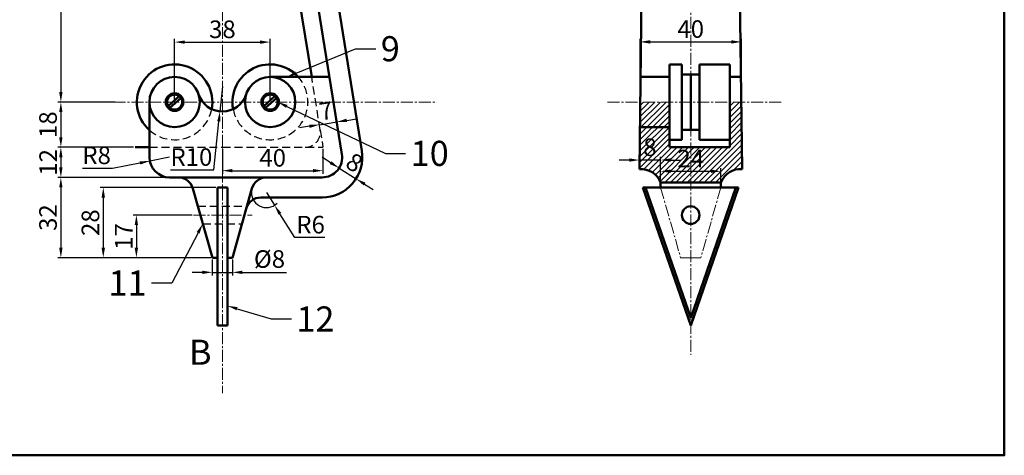
# Model space of a CAD drawing. Units: millimetres. Extents: x 376 to 1043, y -28 to 427.
# Tile 4 of 5: x 651 to 1043, y -28 to 145. Entities that reach past the tile are written whole.
import ezdxf
from ezdxf import colors
from ezdxf.entities.mleader import LeaderData, LeaderLine
from ezdxf.math import Vec2, Vec3

# ---------------------------------------------------------------- set-up
doc = ezdxf.new("R2010")
doc.units = ezdxf.units.MM
doc.header["$LTSCALE"] = 0.5
doc.linetypes.add('CENTER2', pattern=[28.575, 19.05, -3.175, 3.175, -3.175])
doc.linetypes.add('DASHED', pattern=[19.05, 12.7, -6.35])
for name, color, linetype, lineweight in [('M-CNTR', 1, 'CENTER2', 18), ('M-DIMS', 2, 'Continuous', 25), ('M-HATC', 8, 'Continuous', 18), ('M-HIDN', 4, 'DASHED', 25), ('M-OUTL', 7, 'Continuous', 50), ('M-TEXT', 7, 'Continuous', 25)]:
    doc.layers.add(name, color=color, linetype=linetype, lineweight=lineweight)
doc.styles.get("Standard").update_dxf_attribs({"font": 'arial.ttf'})
doc.dimstyles.new('ISO-25', dxfattribs={"dimtxt": 7, "dimasz": 4, "dimexe": 1.25, "dimexo": 0.625, "dimtad": 1, "dimtoh": 1, "dimtxsty": 'Standard', "dimcen": 2.5, "dimadec": 0, "dimazin": 0, "dimtfac": 1, "dimtmove": 0, "dimatfit": 3, "dimfxl": 1, "dimarcsym": 0})

# ---------------------------------------------------------------- blocks, each defined once
blk = doc.blocks.new('*D63')
at = {"layer": 'Defpoints', "color": 0, "ltscale": 0.5, "transparency": 16777216}
for p in [(689.88, 200.26), (667.7, 112.26), (689.88, 112.26)]:
    blk.add_point(p, dxfattribs=at)
at = {"layer": 'M-DIMS', "color": 0, "lineweight": -2, "ltscale": 0.5, "transparency": 16777216}
for p, q in [((689.26, 200.26), (666.45, 200.26)), ((667.7, 196.26), (667.7, 116.26)), ((689.26, 112.26), (666.45, 112.26))]:
    blk.add_line(p, q, dxfattribs=at)
at = {"layer": 'M-DIMS', "color": 0, "ltscale": 0.5, "transparency": 16777216}
for points in [[(667.03, 196.26), (668.37, 196.26), (667.7, 200.26)], [(667.03, 116.26), (668.37, 116.26), (667.7, 112.26)]]:
    blk.add_solid(points, dxfattribs=at)
at = {"layer": 'M-DIMS', "color": 0, "ltscale": 0.5, "transparency": 16777216, "insert": (663.5, 156.26), "char_height": 7, "attachment_point": 5, "rotation": 90}
blk.add_mtext('88', dxfattribs=at)
blk = doc.blocks.new('*D64')
at = {"layer": 'Defpoints', "color": 0, "ltscale": 0.5, "transparency": 16777216}
for p in [(689.88, 112.26), (667.7, 94.26), (697.2, 94.26)]:
    blk.add_point(p, dxfattribs=at)
at = {"layer": 'M-DIMS', "color": 0, "lineweight": -2, "ltscale": 0.5, "transparency": 16777216}
for p, q in [((689.26, 112.26), (666.45, 112.26)), ((667.7, 108.26), (667.7, 98.26)), ((696.58, 94.26), (666.45, 94.26))]:
    blk.add_line(p, q, dxfattribs=at)
at = {"layer": 'M-DIMS', "color": 0, "ltscale": 0.5, "transparency": 16777216}
for points in [[(667.03, 108.26), (668.37, 108.26), (667.7, 112.26)], [(667.03, 98.26), (668.37, 98.26), (667.7, 94.26)]]:
    blk.add_solid(points, dxfattribs=at)
at = {"layer": 'M-DIMS', "color": 0, "ltscale": 0.5, "transparency": 16777216, "insert": (663.5, 103.26), "char_height": 7, "attachment_point": 5, "rotation": 90}
blk.add_mtext('18', dxfattribs=at)
blk = doc.blocks.new('*D65')
at = {"layer": 'Defpoints', "color": 0, "ltscale": 0.5, "transparency": 16777216}
for p in [(691.58, 94.26), (667.7, 82.26), (724.71, 82.26)]:
    blk.add_point(p, dxfattribs=at)
at = {"layer": 'M-DIMS', "color": 0, "lineweight": -2, "ltscale": 0.5, "transparency": 16777216}
for p, q in [((690.96, 94.26), (666.45, 94.26)), ((667.7, 90.26), (667.7, 86.26)), ((724.08, 82.26), (666.45, 82.26))]:
    blk.add_line(p, q, dxfattribs=at)
at = {"layer": 'M-DIMS', "color": 0, "ltscale": 0.5, "transparency": 16777216}
for points in [[(667.03, 90.26), (668.37, 90.26), (667.7, 94.26)], [(667.03, 86.26), (668.37, 86.26), (667.7, 82.26)]]:
    blk.add_solid(points, dxfattribs=at)
at = {"layer": 'M-DIMS', "color": 0, "ltscale": 0.5, "transparency": 16777216, "insert": (663.56, 88.26), "char_height": 7, "attachment_point": 5, "rotation": 90}
blk.add_mtext('12', dxfattribs=at)
blk = doc.blocks.new('*D66')
at = {"layer": 'Defpoints', "color": 0, "ltscale": 0.5, "transparency": 16777216}
for p in [(684.99, 82.26), (667.7, 50.26), (727.94, 50.26)]:
    blk.add_point(p, dxfattribs=at)
at = {"layer": 'M-DIMS', "color": 0, "lineweight": -2, "ltscale": 0.5, "transparency": 16777216}
for p, q in [((684.37, 82.26), (666.45, 82.26)), ((667.7, 78.26), (667.7, 54.26)), ((727.32, 50.26), (666.45, 50.26))]:
    blk.add_line(p, q, dxfattribs=at)
at = {"layer": 'M-DIMS', "color": 0, "ltscale": 0.5, "transparency": 16777216}
for points in [[(667.03, 78.26), (668.37, 78.26), (667.7, 82.26)], [(667.03, 54.26), (668.37, 54.26), (667.7, 50.26)]]:
    blk.add_solid(points, dxfattribs=at)
at = {"layer": 'M-DIMS', "color": 0, "ltscale": 0.5, "transparency": 16777216, "insert": (663.5, 66.26), "char_height": 7, "attachment_point": 5, "rotation": 90}
blk.add_mtext('32', dxfattribs=at)
blk = doc.blocks.new('*D67')
at = {"layer": 'Defpoints', "color": 0, "ltscale": 0.5, "transparency": 16777216}
for p in [(729.94, 78.26), (684.57, 50.26), (717.58, 50.26)]:
    blk.add_point(p, dxfattribs=at)
at = {"layer": 'M-DIMS', "color": 0, "lineweight": -2, "ltscale": 0.5, "transparency": 16777216}
for p, q in [((729.32, 78.26), (683.32, 78.26)), ((684.57, 74.26), (684.57, 54.26)), ((716.96, 50.26), (683.32, 50.26))]:
    blk.add_line(p, q, dxfattribs=at)
at = {"layer": 'M-DIMS', "color": 0, "ltscale": 0.5, "transparency": 16777216}
for points in [[(683.9, 74.26), (685.24, 74.26), (684.57, 78.26)], [(683.9, 54.26), (685.24, 54.26), (684.57, 50.26)]]:
    blk.add_solid(points, dxfattribs=at)
at = {"layer": 'M-DIMS', "color": 0, "ltscale": 0.5, "transparency": 16777216, "insert": (680.37, 64.26), "char_height": 7, "attachment_point": 5, "rotation": 90}
blk.add_mtext('28', dxfattribs=at)
blk = doc.blocks.new('*D68')
at = {"layer": 'Defpoints', "color": 0, "ltscale": 0.5, "transparency": 16777216}
for p in [(720.49, 67.26), (697.74, 50.26), (717.58, 50.26)]:
    blk.add_point(p, dxfattribs=at)
at = {"layer": 'M-DIMS', "color": 0, "lineweight": -2, "ltscale": 0.5, "transparency": 16777216}
for p, q in [((719.87, 67.26), (696.49, 67.26)), ((697.74, 63.26), (697.74, 54.26)), ((716.96, 50.26), (696.49, 50.26))]:
    blk.add_line(p, q, dxfattribs=at)
at = {"layer": 'M-DIMS', "color": 0, "ltscale": 0.5, "transparency": 16777216}
for points in [[(697.07, 63.26), (698.4, 63.26), (697.74, 67.26)], [(697.07, 54.26), (698.4, 54.26), (697.74, 50.26)]]:
    blk.add_solid(points, dxfattribs=at)
at = {"layer": 'M-DIMS', "color": 0, "ltscale": 0.5, "transparency": 16777216, "insert": (693.6, 58.76), "char_height": 7, "attachment_point": 5, "rotation": 90}
blk.add_mtext('17', dxfattribs=at)
blk = doc.blocks.new('*D69')
at = {"layer": 'Defpoints', "color": 0, "ltscale": 0.5, "transparency": 16777216}
for p in [(727.94, 50.26), (735.94, 50.26), (735.94, 44.47)]:
    blk.add_point(p, dxfattribs=at)
at = {"layer": 'M-DIMS', "color": 0, "lineweight": -2, "ltscale": 0.5, "transparency": 16777216}
for p, q in [((727.94, 49.64), (727.94, 43.22)), ((735.94, 49.64), (735.94, 43.22)), ((723.94, 44.47), (719.94, 44.47)), ((727.94, 44.47), (735.94, 44.47)), ((739.94, 44.47), (757.41, 44.47))]:
    blk.add_line(p, q, dxfattribs=at)
at = {"layer": 'M-DIMS', "color": 0, "ltscale": 0.5, "transparency": 16777216}
for points in [[(723.94, 45.14), (723.94, 43.8), (727.94, 44.47)], [(739.94, 45.14), (739.94, 43.8), (735.94, 44.47)]]:
    blk.add_solid(points, dxfattribs=at)
at = {"layer": 'M-DIMS', "color": 0, "ltscale": 0.5, "transparency": 16777216, "insert": (750.68, 48.87), "char_height": 7, "attachment_point": 5}
blk.add_mtext('%%C8', dxfattribs=at)
blk = doc.blocks.new('*D70')
at = {"layer": 'Defpoints', "color": 0, "ltscale": 0.5, "transparency": 16777216}
for p in [(710.94, 90.26), (703.08, 88.78)]:
    blk.add_point(p, dxfattribs=at)
at = {"layer": 'M-DIMS', "color": 0, "lineweight": -2, "ltscale": 0.5, "transparency": 16777216}
for p, q in [((710.94, 90.26), (703.08, 88.78)), ((688.2, 85.96), (699.15, 88.03)), ((676.27, 85.96), (688.2, 85.96))]:
    blk.add_line(p, q, dxfattribs=at)
at = {"layer": 'M-DIMS', "color": 0, "ltscale": 0.5, "transparency": 16777216}
blk.add_solid([(699.03, 88.69), (699.28, 87.38), (703.08, 88.78)], dxfattribs=at)
at = {"layer": 'M-DIMS', "color": 0, "ltscale": 0.5, "transparency": 16777216, "insert": (681.92, 90.16), "char_height": 7, "attachment_point": 5}
blk.add_mtext('R8', dxfattribs=at)
blk = doc.blocks.new('*D71')
at = {"layer": 'Defpoints', "color": 0, "ltscale": 0.5, "transparency": 16777216}
for p in [(731.94, 94.26), (771.94, 94.26), (771.94, 84.95)]:
    blk.add_point(p, dxfattribs=at)
at = {"layer": 'M-DIMS', "color": 0, "lineweight": -2, "ltscale": 0.5, "transparency": 16777216}
for p, q in [((731.94, 93.64), (731.94, 83.7)), ((771.94, 93.64), (771.94, 83.7)), ((735.94, 84.95), (767.94, 84.95))]:
    blk.add_line(p, q, dxfattribs=at)
at = {"layer": 'M-DIMS', "color": 0, "ltscale": 0.5, "transparency": 16777216}
for points in [[(735.94, 85.61), (735.94, 84.28), (731.94, 84.95)], [(767.94, 85.61), (767.94, 84.28), (771.94, 84.95)]]:
    blk.add_solid(points, dxfattribs=at)
at = {"layer": 'M-DIMS', "color": 0, "ltscale": 0.5, "transparency": 16777216, "insert": (751.94, 89.15), "char_height": 7, "attachment_point": 5}
blk.add_mtext('40', dxfattribs=at)
blk = doc.blocks.new('*D72')
at = {"layer": 'Defpoints', "color": 0, "ltscale": 0.5, "transparency": 16777216}
for p in [(750.94, 136.13), (712.94, 112.26), (750.94, 112.26)]:
    blk.add_point(p, dxfattribs=at)
at = {"layer": 'M-DIMS', "color": 0, "lineweight": -2, "ltscale": 0.5, "transparency": 16777216}
for p, q in [((712.94, 112.89), (712.94, 137.38)), ((750.94, 112.89), (750.94, 137.38)), ((716.94, 136.13), (746.94, 136.13))]:
    blk.add_line(p, q, dxfattribs=at)
at = {"layer": 'M-DIMS', "color": 0, "ltscale": 0.5, "transparency": 16777216}
for points in [[(716.94, 136.79), (716.94, 135.46), (712.94, 136.13)], [(746.94, 136.79), (746.94, 135.46), (750.94, 136.13)]]:
    blk.add_solid(points, dxfattribs=at)
at = {"layer": 'M-DIMS', "color": 0, "ltscale": 0.5, "transparency": 16777216, "insert": (731.94, 140.33), "char_height": 7, "attachment_point": 5}
blk.add_mtext('38', dxfattribs=at)
blk = doc.blocks.new('*D73')
at = {"layer": 'Defpoints', "color": 0, "ltscale": 0.5, "transparency": 16777216}
for p in [(731.94, 118.51), (730.94, 108.56)]:
    blk.add_point(p, dxfattribs=at)
at = {"layer": 'M-DIMS', "color": 0, "lineweight": -2, "ltscale": 0.5, "transparency": 16777216}
for p, q in [((731.94, 118.51), (730.94, 108.56)), ((728.6, 85.26), (730.54, 104.58)), ((711.27, 85.26), (728.6, 85.26))]:
    blk.add_line(p, q, dxfattribs=at)
at = {"layer": 'M-DIMS', "color": 0, "ltscale": 0.5, "transparency": 16777216}
blk.add_solid([(729.88, 104.65), (731.2, 104.51), (730.94, 108.56)], dxfattribs=at)
at = {"layer": 'M-DIMS', "color": 0, "ltscale": 0.5, "transparency": 16777216, "insert": (719.62, 89.45), "char_height": 7, "attachment_point": 5}
blk.add_mtext('R10', dxfattribs=at)
blk = doc.blocks.new('*D74')
at = {"layer": 'Defpoints', "color": 0, "ltscale": 0.5, "transparency": 16777216}
for p in [(778.34, 86), (785.11, 81.73), (785.11, 81.73)]:
    blk.add_point(p, dxfattribs=at)
at = {"layer": 'M-DIMS', "color": 0, "lineweight": -2, "ltscale": 0.5, "transparency": 16777216}
for p, q in [((774.96, 88.13), (771.57, 90.26)), ((778.01, 85.47), (777.67, 84.94)), ((778.34, 86), (785.11, 81.73)), ((785.44, 82.26), (785.77, 82.79)), ((788.49, 79.6), (791.87, 77.47))]:
    blk.add_line(p, q, dxfattribs=at)
at = {"layer": 'M-DIMS', "color": 0, "ltscale": 0.5, "transparency": 16777216}
for points in [[(775.31, 88.7), (774.6, 87.57), (778.34, 86)], [(788.85, 80.16), (788.14, 79.04), (785.11, 81.73)]]:
    blk.add_solid(points, dxfattribs=at)
at = {"layer": 'M-DIMS', "color": 0, "ltscale": 0.5, "transparency": 16777216, "insert": (783.96, 87.42), "char_height": 7, "attachment_point": 5, "rotation": 327.7752}
blk.add_mtext('8', dxfattribs=at)
blk = doc.blocks.new('*D75')
at = {"layer": 'Defpoints', "color": 0, "ltscale": 0.5, "transparency": 16777216}
for p in [(770.5, 103.23), (777.42, 104.34), (777.42, 104.34)]:
    blk.add_point(p, dxfattribs=at)
at = {"layer": 'M-DIMS', "color": 0, "lineweight": -2, "ltscale": 0.5, "transparency": 16777216}
for p, q in [((766.56, 102.6), (762.61, 101.96)), ((770.41, 103.85), (770.31, 104.46)), ((770.5, 103.23), (777.42, 104.34)), ((777.32, 104.96), (777.22, 105.57)), ((781.37, 104.97), (785.32, 105.61))]:
    blk.add_line(p, q, dxfattribs=at)
at = {"layer": 'M-DIMS', "color": 0, "ltscale": 0.5, "transparency": 16777216}
for points in [[(766.45, 103.25), (766.66, 101.94), (770.5, 103.23)], [(781.26, 105.63), (781.47, 104.31), (777.42, 104.34)]]:
    blk.add_solid(points, dxfattribs=at)
at = {"layer": 'M-DIMS', "color": 0, "ltscale": 0.5, "transparency": 16777216, "insert": (773.31, 107.86), "char_height": 7, "attachment_point": 5, "rotation": 9.1114}
blk.add_mtext('7', dxfattribs=at)
blk = doc.blocks.new('*D81')
at = {"layer": 'Defpoints', "color": 0, "ltscale": 0.5, "transparency": 16777216}
for p in [(749.49, 76.26), (752.68, 71.19)]:
    blk.add_point(p, dxfattribs=at)
at = {"layer": 'M-DIMS', "color": 0, "lineweight": -2, "ltscale": 0.5, "transparency": 16777216}
for p, q in [((749.49, 76.26), (752.68, 71.19)), ((760.75, 58.36), (754.81, 67.8)), ((772.66, 58.36), (760.75, 58.36))]:
    blk.add_line(p, q, dxfattribs=at)
blk.add_arc((749.49, 76.26), 6, 170.2597, 314.1138, dxfattribs=at)
at = {"layer": 'M-DIMS', "color": 0, "ltscale": 0.5, "transparency": 16777216}
blk.add_solid([(755.38, 68.16), (754.25, 67.45), (752.68, 71.19)], dxfattribs=at)
at = {"layer": 'M-DIMS', "color": 0, "ltscale": 0.5, "transparency": 16777216, "insert": (767.02, 62.56), "char_height": 7, "attachment_point": 5}
blk.add_mtext('R6', dxfattribs=at)
blk = doc.blocks.new('*D85')
at = {"layer": 'Defpoints', "color": 0, "ltscale": 0.5, "transparency": 16777216}
for p in [(930.2, 84.71), (906.2, 78.26), (930.2, 78.26)]:
    blk.add_point(p, dxfattribs=at)
at = {"layer": 'M-DIMS', "color": 0, "lineweight": -2, "ltscale": 0.5, "transparency": 16777216}
for p, q in [((906.2, 78.89), (906.2, 85.96)), ((910.2, 84.71), (926.2, 84.71)), ((930.2, 78.89), (930.2, 85.96))]:
    blk.add_line(p, q, dxfattribs=at)
at = {"layer": 'M-DIMS', "color": 0, "ltscale": 0.5, "transparency": 16777216}
for points in [[(910.2, 85.38), (910.2, 84.04), (906.2, 84.71)], [(926.2, 85.38), (926.2, 84.04), (930.2, 84.71)]]:
    blk.add_solid(points, dxfattribs=at)
at = {"layer": 'M-DIMS', "color": 0, "ltscale": 0.5, "transparency": 16777216, "insert": (918.2, 88.85), "char_height": 7, "attachment_point": 5}
blk.add_mtext('24', dxfattribs=at)
blk = doc.blocks.new('*D86')
at = {"layer": 'Defpoints', "color": 0, "ltscale": 0.5, "transparency": 16777216}
for p in [(897.77, 89.18), (897.77, 85.57), (906.2, 80.26)]:
    blk.add_point(p, dxfattribs=at)
at = {"layer": 'M-DIMS', "color": 0, "lineweight": -2, "ltscale": 0.5, "transparency": 16777216}
for p, q in [((897.77, 86.19), (897.77, 90.43)), ((906.2, 80.89), (906.2, 90.43)), ((893.77, 89.18), (889.77, 89.18)), ((906.2, 89.18), (897.77, 89.18)), ((910.2, 89.18), (914.2, 89.18))]:
    blk.add_line(p, q, dxfattribs=at)
at = {"layer": 'M-DIMS', "color": 0, "ltscale": 0.5, "transparency": 16777216}
for points in [[(893.77, 89.85), (893.77, 88.52), (897.77, 89.18)], [(910.2, 89.85), (910.2, 88.52), (906.2, 89.18)]]:
    blk.add_solid(points, dxfattribs=at)
at = {"layer": 'M-DIMS', "color": 0, "ltscale": 0.5, "transparency": 16777216, "insert": (901.99, 93.38), "char_height": 7, "attachment_point": 5}
blk.add_mtext('8', dxfattribs=at)
blk = doc.blocks.new('*D87')
at = {"layer": 'Defpoints', "color": 0, "ltscale": 0.5, "transparency": 16777216}
for p in [(938.33, 136.22), (898.08, 112.26), (938.33, 112.82)]:
    blk.add_point(p, dxfattribs=at)
at = {"layer": 'M-DIMS', "color": 0, "lineweight": -2, "ltscale": 0.5, "transparency": 16777216}
for p, q in [((898.08, 112.89), (898.08, 137.47)), ((938.33, 113.44), (938.33, 137.47)), ((902.08, 136.22), (934.33, 136.22))]:
    blk.add_line(p, q, dxfattribs=at)
at = {"layer": 'M-DIMS', "color": 0, "ltscale": 0.5, "transparency": 16777216}
for points in [[(902.08, 136.89), (902.08, 135.55), (898.08, 136.22)], [(934.33, 136.89), (934.33, 135.55), (938.33, 136.22)]]:
    blk.add_solid(points, dxfattribs=at)
at = {"layer": 'M-DIMS', "color": 0, "ltscale": 0.5, "transparency": 16777216, "insert": (918.2, 140.42), "char_height": 7, "attachment_point": 5}
blk.add_mtext('40', dxfattribs=at)

msp = doc.modelspace()

# ---------------------------------------------------------------- hatches: boundary and pattern name
at = {"layer": 'M-HATC', "ltscale": 0.5}
h = msp.add_hatch(dxfattribs=at)
h.set_pattern_fill('ANSI31', color=256, scale=0.5)
h.set_pattern_definition([(45, (1108.3857, -159.2338), (-1.122532, 1.122532), [])])
h.paths.add_polyline_path([(918.196, 94.264), (909.696, 94.264), (909.696, 97.264), (909.696, 112.264), (898.081, 112.264), (897.774, 85.565, -0.3292722), (906.196, 80.264), (918.196, 80.264)])
h.paths.add_polyline_path([(938.334, 112.264), (933.696, 112.264), (933.696, 97.264), (933.696, 94.264), (918.196, 94.264), (918.196, 80.264), (930.196, 80.264, -0.332046), (938.703, 85.559)])

# ---------------------------------------------------------------- linework, layer by layer
at = {"layer": 'M-CNTR', "ltscale": 0.5}
for p, q in [((731.943, 320.737), (731.943, -3.612)), ((918.196, 160.434), (918.196, 11.662)), ((681.456, 112.264), (817.274, 112.264)), ((885.063, 112.264), (954.37, 112.264)), ((906.196, 78.264), (914.196, 50.264)), ((930.196, 78.264), (922.196, 50.264)), ((720.493, 67.264), (743.745, 67.264)), ((918.196, 50.264), (914.196, 50.264)), ((918.196, 50.264), (922.196, 50.264))]:
    msp.add_line(p, q, dxfattribs=at)
at = {"layer": 'M-HIDN', "ltscale": 0.5}
for p, q in [((770.828, 101.214), (767.452, 122.264)), ((770.828, 101.214), (771.943, 94.264)), ((702.943, 94.264), (731.943, 94.264)), ((731.943, 94.264), (771.943, 94.264)), ((722.177, 70.764), (741.708, 70.764)), ((724.146, 63.764), (739.739, 63.764))]:
    msp.add_line(p, q, dxfattribs=at)
for centre, radius, start, end in [((750.943, 112.264), 15, 190.76015, 41.81031), ((712.943, 112.264), 15, 228.18969, 349.23985), ((764.904, 100.264), 6, 270, 9.11136)]:
    msp.add_arc(centre, radius, start, end, dxfattribs=at)
at = {"layer": 'M-OUTL', "ltscale": 0.5}
for p, q in [((754.943, 200.264), (767.452, 122.264)), ((899.107, 201.264), (897.774, 85.565)), ((937.107, 201.264), (938.703, 85.559)), ((909.696, 127.264), (909.696, 97.264)), ((914.696, 127.264), (909.696, 127.264)), ((914.696, 123.264), (914.696, 127.264)), ((933.696, 127.264), (921.696, 127.264)), ((921.696, 127.264), (921.696, 123.264)), ((933.696, 97.264), (933.696, 127.264)), ((750.943, 122.264), (774.541, 122.264)), ((898.196, 122.264), (909.696, 122.264)), ((914.696, 97.264), (914.696, 123.264)), ((921.696, 123.264), (914.696, 123.264)), ((918.196, 123.264), (918.196, 101.264)), ((921.696, 123.264), (921.696, 97.264)), ((938.196, 122.264), (933.696, 122.264)), ((710.408, 110.659), (714.809, 114.613)), ((711.076, 109.915), (715.477, 113.869)), ((748.408, 110.659), (752.809, 114.613)), ((749.076, 109.915), (753.477, 113.869)), ((702.943, 112.264), (702.943, 90.264)), ((898.196, 102.264), (909.696, 102.264)), ((914.696, 101.264), (921.696, 101.264)), ((702.943, 94.264), (697.204, 94.264)), ((909.696, 97.264), (914.696, 97.264)), ((909.696, 97.264), (909.696, 94.264)), ((909.696, 94.264), (933.696, 94.264)), ((921.696, 97.264), (933.696, 97.264)), ((933.696, 97.264), (933.696, 94.264)), ((771.571, 82.264), (710.943, 82.264)), ((906.196, 78.264), (906.196, 80.264)), ((906.196, 80.264), (930.196, 80.264)), ((930.196, 80.264), (930.196, 78.264)), ((727.943, 50.264), (720.173, 77.889)), ((731.943, 78.264), (729.943, 78.264)), ((729.943, 23.264), (729.943, 78.264)), ((731.943, 78.264), (733.943, 78.264)), ((733.943, 78.264), (733.943, 23.264)), ((735.943, 50.264), (743.712, 77.889)), ((899.196, 78.264), (937.196, 78.264)), ((918.196, 23.264), (899.196, 78.264)), ((899.196, 78.264), (937.196, 78.264)), ((918.196, 26.327), (900.254, 78.264)), ((918.196, 23.264), (937.196, 78.264)), ((918.196, 26.327), (936.138, 78.264)), ((771.571, 74.264), (747.238, 74.264)), ((729.943, 50.264), (727.943, 50.264)), ((733.943, 50.264), (735.943, 50.264)), ((733.943, 23.264), (729.943, 23.264))]:
    msp.add_line(p, q, dxfattribs=at)
msp.add_lwpolyline([(376.448, 426.986), (1042.916, 426.986), (1042.916, -28.377), (376.448, -28.377)], close=True, dxfattribs=at)
for points in [[(753.943, 215.264), (754.09, 215.264, -0.3683676), (769.888, 201.798), (787.369, 92.798, -0.4615956), (771.571, 74.264)], [(732.986, 207.264), (754.09, 207.264, -0.3683676), (761.989, 200.531), (779.47, 91.531, -0.4615956), (771.571, 82.264)]]:
    msp.add_lwpolyline(points, format="xyb", dxfattribs=at)
for centre, radius in [((712.943, 112.264), 10), ((750.943, 112.264), 10), ((712.943, 112.264), 3.5), ((712.943, 112.264), 3), ((750.943, 112.264), 3.5), ((750.943, 112.264), 3), ((918.196, 67.264), 3.5)]:
    msp.add_circle(centre, radius, dxfattribs=at)
for centre, radius, start, end in [((712.943, 112.264), 15, 349.23985, 228.18969), ((750.943, 112.264), 15, 41.81031, 190.76015), ((731.943, 118.509), 10, 198.19487, 341.80513), ((710.943, 90.264), 8, 180, 270), ((714.397, 76.264), 6, 15.70864, 90), ((749.488, 76.264), 6, 90, 164.29136), ((898.396, 77.213), 8.376, 21.36356, 94.26468), ((937.996, 77.213), 8.376, 85.16227, 158.63644), ((747.238, 68.264), 6, 90, 164.29136)]:
    msp.add_arc(centre, radius, start, end, dxfattribs=at)

# ---------------------------------------------------------------- texts
at = {"layer": 'M-TEXT', "ltscale": 0.5, "insert": (718.665, 17.665), "char_height": 10, "attachment_point": 1}
msp.add_mtext_dynamic_manual_height_columns('B', width=13.27748, gutter_width=12.5, heights=[0], dxfattribs=at)

# ---------------------------------------------------------------- dimensions: what is measured, and where the dimension line sits
at = {"layer": 'M-DIMS', "ltscale": 0.5}
for base, p1, p2, picture, middle in [((667.699, 112.264), (689.883, 200.264), (689.883, 112.264), '*D63', (663.5, 156.264)), ((667.699, 94.264), (689.883, 112.264), (697.204, 94.264), '*D64', (663.5, 103.264)), ((667.699, 82.264), (691.585, 94.264), (724.706, 82.264), '*D65', (663.559, 88.264)), ((667.699, 50.264), (684.991, 82.264), (727.943, 50.264), '*D66', (663.497, 66.264)), ((684.571, 50.264), (729.943, 78.264), (717.584, 50.264), '*D67', (680.372, 64.264)), ((697.738, 50.264), (720.493, 67.264), (717.584, 50.264), '*D68', (693.599, 58.764))]:
    dim = msp.add_linear_dim(base=base, p1=p1, p2=p2, angle=90, dimstyle='ISO-25', override={"dimclrd": 0, "dimclre": 0, "dimclrt": 0}, dxfattribs=at)
    dim.commit()
    dim.dimension.update_dxf_attribs({"geometry": picture, "text_midpoint": middle})
for base, p1, p2, picture, middle in [((750.943, 136.127), (712.943, 112.264), (750.943, 112.264), '*D72', (731.943, 140.329)), ((771.943, 84.946), (731.943, 94.264), (771.943, 94.264), '*D71', (751.943, 89.145)), ((930.196, 84.712), (906.196, 78.264), (930.196, 78.264), '*D85', (918.196, 88.851))]:
    dim = msp.add_linear_dim(base=base, p1=p1, p2=p2, dimstyle='ISO-25', override={"dimclrd": 0, "dimclre": 0, "dimclrt": 0}, dxfattribs=at)
    dim.commit()
    dim.dimension.update_dxf_attribs({"geometry": picture, "text_midpoint": middle})
for base, p1, p2, text, picture, middle in [((938.327, 136.22), (898.081, 112.264), (938.327, 112.819), '40', '*D87', (918.204, 140.419)), ((897.774, 89.185), (906.196, 80.264), (897.774, 85.565), '8', '*D86', (901.985, 93.384))]:
    dim = msp.add_linear_dim(base=base, p1=p1, p2=p2, text=text, dimstyle='ISO-25', override={"dimclrd": 0, "dimclre": 0, "dimclrt": 0}, dxfattribs=at)
    dim.commit()
    dim.dimension.update_dxf_attribs({"geometry": picture, "text_midpoint": middle})
dim = msp.add_radius_dim(center=(731.943, 118.509), mpoint=(730.942, 108.559), dimstyle='ISO-25', override={"dimclrd": 0, "dimclre": 0, "dimclrt": 0}, dxfattribs=at)
dim.commit()
dim.dimension.update_dxf_attribs({"geometry": '*D73', "text_midpoint": (719.621, 85.256), "dimtype": 164})
for p1, p2, picture, middle in [((770.505, 103.23), (777.416, 104.339), '*D75', (773.307, 107.857)), ((778.339, 85.998), (785.107, 81.732), '*D74', (783.962, 87.418))]:
    dim = msp.add_aligned_dim(p1=p1, p2=p2, distance=0, dimstyle='ISO-25', override={"dimclrd": 0, "dimclre": 0, "dimclrt": 0}, dxfattribs=at)
    dim.commit()
    dim.dimension.update_dxf_attribs({"geometry": picture, "text_midpoint": middle})
for center, mpoint, picture, middle in [((710.943, 90.264), (703.082, 88.776), '*D70', (681.923, 90.156)), ((749.488, 76.264), (752.683, 71.186), '*D81', (767.017, 62.563))]:
    dim = msp.add_radius_dim(center=center, mpoint=mpoint, dimstyle='ISO-25', override={"dimclrd": 0, "dimclre": 0, "dimclrt": 0}, dxfattribs=at)
    dim.commit()
    dim.dimension.update_dxf_attribs({"geometry": picture, "text_midpoint": middle})
dim = msp.add_linear_dim(base=(735.943, 44.47), p1=(727.943, 50.264), p2=(735.943, 50.264), text='%%C<>', dimstyle='ISO-25', override={"dimclrd": 0, "dimclre": 0, "dimclrt": 0}, dxfattribs=at)
dim.commit()
dim.dimension.update_dxf_attribs({"geometry": '*D69', "text_midpoint": (750.677, 44.47), "dimtype": 160})

# ---------------------------------------------------------------- leaders
ml = msp.add_multileader_mtext('Standard', dxfattribs=at)
ml.set_content('9', color=256)
ml.set_leader_properties()
ml.build(insert=Vec2(0, 0))
ctx = ml.context
ctx.base_point, ctx.char_height, ctx.plane_origin = Vec3(792.933, 133.399), 10, Vec3(757.551, 122.264)
notes = []
notes.append((ctx, [(0, (1, 1, 0), (784.933, 133.399), (1, 0), 8, [(0, [(757.551, 122.264)], 0, [])])]))
ctx.mtext.insert, ctx.mtext.flow_direction = Vec3(794.933, 138.485), 5
ml = msp.add_multileader_mtext('Standard', dxfattribs=at)
ml.set_content('10', color=256)
ml.set_leader_properties()
ml.build(insert=Vec2(0, 0))
ctx = ml.context
ctx.base_point, ctx.char_height, ctx.plane_origin = Vec3(804.827, 91.748), 10, Vec3(753.943, 112.264)
notes.append((ctx, [(0, (1, 1, 0), (796.827, 91.748), (1, 0), 8, [(0, [(753.943, 112.264)], 0, [])])]))
ctx.mtext.insert, ctx.mtext.flow_direction = Vec3(806.827, 96.833), 5
ml = msp.add_multileader_mtext('Standard', dxfattribs=at)
ml.set_content('11', color=256)
ml.set_leader_properties()
ml.build(insert=Vec2(0, 0))
ctx = ml.context
ctx.base_point, ctx.char_height, ctx.plane_origin = Vec3(688.328, 40.214), 10, Vec3(724.146, 63.764)
ctx.text_align_type = 2
notes.append((ctx, [(0, (1, 1, 0), (711.781, 40.214), (-1, 0), 8, [(0, [(724.146, 63.764)], 0, [])])]))
ctx.mtext.insert, ctx.mtext.alignment, ctx.mtext.flow_direction = Vec3(701.781, 45.214), 3, 5
ml = msp.add_multileader_mtext('Standard', dxfattribs=at)
ml.set_content('12', color=256)
ml.set_leader_properties()
ml.build(insert=Vec2(0, 0))
ctx = ml.context
ctx.base_point, ctx.char_height, ctx.plane_origin = Vec3(759.368, 25.912), 10, Vec3(733.943, 31.141)
notes.append((ctx, [(0, (1, 1, 0), (751.368, 25.912), (1, 0), 8, [(0, [(733.943, 31.141)], 0, [])])]))
ctx.mtext.insert, ctx.mtext.flow_direction = Vec3(761.368, 30.912), 5
for ctx, leaders in notes:
    for number, flags, end, landing, length, lines in leaders:
        leader = LeaderData()
        leader.index, (leader.has_last_leader_line, leader.has_dogleg_vector, leader.attachment_direction) = number, flags
        leader.last_leader_point, leader.dogleg_vector, leader.dogleg_length = Vec3(end), Vec3(landing), length
        for number, points, colour, breaks in lines:
            line = LeaderLine()
            line.index, line.vertices, line.color, line.breaks = number, Vec3.list(points), colors.encode_raw_color(colour), breaks
            leader.lines.append(line)
        ctx.leaders.append(leader)

doc.saveas('drawing.dxf')
